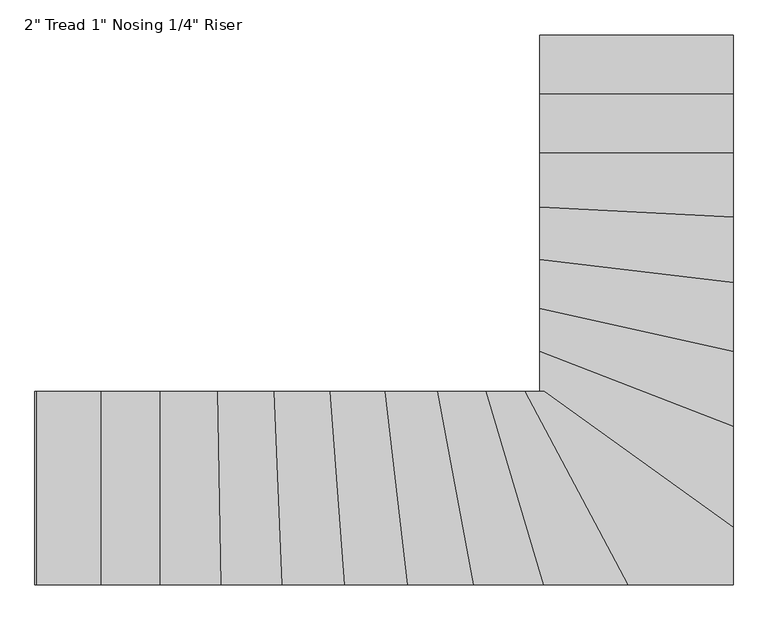
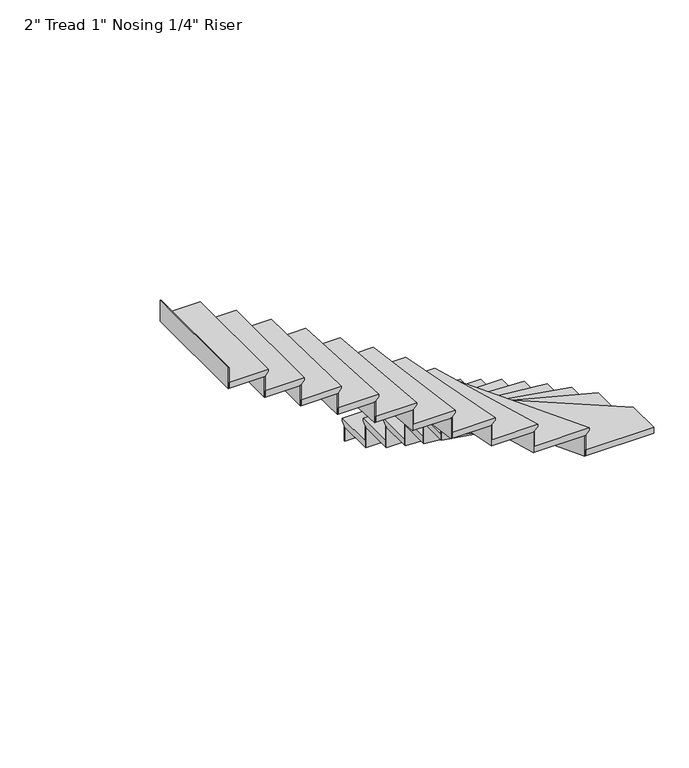
"""IFC4 building model written with IfcOpenShell, lengths in millimetres: stair flight geometry."""

from ifc_helpers import new_model, si_unit, origin, place, context, project, spatial, faceted_brep, source, transform, mapped, element, save


def stair_flight_9178a8c5(model_context):
    return source(origin(), model_context, "Body", "Brep", [
        faceted_brep([(541.8084916, 3870.4222402, 6551.0833333), (541.8084916, 3870.4222402, 6570.1333333), (1456.2084916, 3870.4222402, 6570.1333333), (1456.2084916, 3870.4222402, 6551.0833333), (541.8084916, 3845.0222402, 6525.6833333), (1456.2084916, 3845.0222402, 6525.6833333), (541.8084916, 3565.6222402, 6570.1333333), (1456.2084916, 3565.6222402, 6570.1333333), (1456.2084916, 3845.0222402, 6519.3333333), (1456.2084916, 3565.6222402, 6519.3333333), (541.8084916, 3565.6222402, 6519.3333333), (541.8084916, 3845.0222402, 6519.3333333)], [[[0, 1, 2, 3]], [[4, 0, 3, 5]], [[2, 1, 6, 7]], [[8, 9, 10, 11]], [[2, 7, 9, 8, 5, 3]], [[8, 11, 4, 5]], [[6, 1, 0, 4, 11, 10]], [[7, 6, 10, 9]]]),
        faceted_brep([(541.8084916, 3845.0222402, 6519.3333333), (541.8084916, 3845.0222402, 6400.8), (541.8084916, 3838.6722402, 6400.8), (541.8084916, 3838.6722402, 6519.3333333), (1456.2084916, 3845.0222402, 6519.3333333), (1456.2084916, 3838.6722402, 6519.3333333), (1456.2084916, 3838.6722402, 6400.8), (1456.2084916, 3845.0222402, 6400.8)], [[[0, 1, 2, 3]], [[4, 5, 6, 7]], [[1, 0, 4, 7]], [[2, 1, 7, 6]], [[3, 2, 6, 5]], [[0, 3, 5, 4]]]),
        faceted_brep([(541.8084916, 3565.6222402, 6688.6666667), (541.8084916, 3565.6222402, 6519.3333333), (541.8084916, 3559.2722402, 6519.3333333), (541.8084916, 3559.2722402, 6688.6666667), (1456.2084916, 3565.6222402, 6688.6666667), (1456.2084916, 3559.2722402, 6688.6666667), (1456.2084916, 3559.2722402, 6519.3333333), (1456.2084916, 3565.6222402, 6519.3333333)], [[[0, 1, 2, 3]], [[4, 5, 6, 7]], [[1, 0, 4, 7]], [[2, 1, 7, 6]], [[3, 2, 6, 5]], [[0, 3, 5, 4]]]),
        faceted_brep([(1456.2084916, 3591.0222402, 6739.4666667), (541.8084916, 3591.0222402, 6739.4666667), (541.8084916, 3286.2222402, 6739.4666667), (1456.2084916, 3286.2222402, 6739.4666667), (1456.2084916, 3565.6222402, 6688.6666667), (1456.2084916, 3286.2222402, 6688.6666667), (541.8084916, 3286.2222402, 6688.6666667), (541.8084916, 3565.6222402, 6688.6666667), (1456.2084916, 3565.6222402, 6695.0166667), (1456.2084916, 3591.0222402, 6720.4166667), (541.8084916, 3565.6222402, 6695.0166667), (541.8084916, 3591.0222402, 6720.4166667)], [[[0, 1, 2, 3]], [[4, 5, 6, 7]], [[0, 3, 5, 4, 8, 9]], [[4, 7, 10, 8]], [[2, 1, 11, 10, 7, 6]], [[3, 2, 6, 5]], [[11, 1, 0, 9]], [[10, 11, 9, 8]]]),
        faceted_brep([(541.8084916, 3286.2222402, 6858.0), (541.8084916, 3286.2222402, 6688.6666667), (541.8084916, 3279.8722402, 6688.6666667), (541.8084916, 3279.8722402, 6858.0), (1456.2084916, 3286.2222402, 6858.0), (1456.2084916, 3279.8722402, 6858.0), (1456.2084916, 3279.8722402, 6688.6666667), (1456.2084916, 3286.2222402, 6688.6666667)], [[[0, 1, 2, 3]], [[4, 5, 6, 7]], [[1, 0, 4, 7]], [[2, 1, 7, 6]], [[3, 2, 6, 5]], [[0, 3, 5, 4]]]),
        faceted_brep([(1456.2084916, 3311.6222402, 6908.8), (541.8084916, 3311.6222402, 6908.8), (541.8084916, 3029.9557204, 6908.8), (1456.2084916, 2983.6235901, 6908.8), (1456.2084916, 3286.2222402, 6858.0), (1456.2084916, 2983.6235901, 6858.0), (541.8084916, 3029.9557204, 6858.0), (541.8084916, 3286.2222402, 6858.0), (1456.2084916, 3286.2222402, 6864.35), (1456.2084916, 3311.6222402, 6889.75), (541.8084916, 3286.2222402, 6864.35), (541.8084916, 3311.6222402, 6889.75)], [[[0, 1, 2, 3]], [[4, 5, 6, 7]], [[0, 3, 5, 4, 8, 9]], [[4, 7, 10, 8]], [[2, 1, 11, 10, 7, 6]], [[3, 2, 6, 5]], [[11, 1, 0, 9]], [[10, 11, 9, 8]]]),
        faceted_brep([(541.8084916, 3029.9557204, 7027.3333333), (541.8084916, 3029.9557204, 6858.0), (541.8084916, 3023.5975741, 6858.0), (541.8084916, 3023.5975741, 7027.3333333), (1456.2084916, 2983.6235901, 7027.3333333), (1456.2084916, 2977.2654439, 7027.3333333), (1456.2084916, 2977.2654439, 6858.0), (1456.2084916, 2983.6235901, 6858.0)], [[[0, 1, 2, 3]], [[4, 5, 6, 7]], [[1, 0, 4, 7]], [[2, 1, 7, 6]], [[3, 2, 6, 5]], [[0, 3, 5, 4]]]),
        faceted_brep([(1456.2084916, 3009.0561751, 7078.1333333), (541.8084916, 3055.3883053, 7078.1333333), (541.8084916, 2782.3369776, 7078.1333333), (1456.2084916, 2672.1399389, 7078.1333333), (1456.2084916, 2983.6235901, 7027.3333333), (1456.2084916, 2672.1399389, 7027.3333333), (541.8084916, 2782.3369776, 7027.3333333), (541.8084916, 3029.9557204, 7027.3333333), (1456.2084916, 2983.6235901, 7033.6833333), (1456.2084916, 3009.0561751, 7059.0833333), (541.8084916, 3029.9557204, 7033.6833333), (541.8084916, 3055.3883053, 7059.0833333)], [[[0, 1, 2, 3]], [[4, 5, 6, 7]], [[0, 3, 5, 4, 8, 9]], [[4, 7, 10, 8]], [[2, 1, 11, 10, 7, 6]], [[3, 2, 6, 5]], [[11, 1, 0, 9]], [[10, 11, 9, 8]]]),
        faceted_brep([(541.8084916, 2782.3369776, 7196.6666667), (541.8084916, 2782.3369776, 7027.3333333), (541.8084916, 2775.9410322, 7027.3333333), (541.8084916, 2775.9410322, 7196.6666667), (1456.2084916, 2672.1399389, 7196.6666667), (1456.2084916, 2665.7439934, 7196.6666667), (1456.2084916, 2665.7439934, 7027.3333333), (1456.2084916, 2672.1399389, 7027.3333333)], [[[0, 1, 2, 3]], [[4, 5, 6, 7]], [[1, 0, 4, 7]], [[2, 1, 7, 6]], [[3, 2, 6, 5]], [[0, 3, 5, 4]]]),
        faceted_brep([(1456.2084916, 2697.7237208, 7247.4666667), (541.8084916, 2807.9207596, 7247.4666667), (541.8084916, 2549.3331683, 7247.4666667), (1456.2084916, 2345.4640286, 7247.4666667), (1456.2084916, 2672.1399389, 7196.6666667), (1456.2084916, 2345.4640286, 7196.6666667), (541.8084916, 2549.3331683, 7196.6666667), (541.8084916, 2782.3369776, 7196.6666667), (1456.2084916, 2672.1399389, 7203.0166667), (1456.2084916, 2697.7237208, 7228.4166667), (541.8084916, 2782.3369776, 7203.0166667), (541.8084916, 2807.9207596, 7228.4166667)], [[[0, 1, 2, 3]], [[4, 5, 6, 7]], [[0, 3, 5, 4, 8, 9]], [[4, 7, 10, 8]], [[2, 1, 11, 10, 7, 6]], [[3, 2, 6, 5]], [[11, 1, 0, 9]], [[10, 11, 9, 8]]]),
        faceted_brep([(541.8084916, 2549.3331683, 7366.0), (541.8084916, 2549.3331683, 7196.6666667), (541.8084916, 2542.8272579, 7196.6666667), (541.8084916, 2542.8272579, 7366.0), (1456.2084916, 2345.4640286, 7366.0), (1456.2084916, 2338.9581182, 7366.0), (1456.2084916, 2338.9581182, 7196.6666667), (1456.2084916, 2345.4640286, 7196.6666667)], [[[0, 1, 2, 3]], [[4, 5, 6, 7]], [[1, 0, 4, 7]], [[2, 1, 7, 6]], [[3, 2, 6, 5]], [[0, 3, 5, 4]]]),
        faceted_brep([(1456.2084916, 2371.4876703, 7416.8), (541.8084916, 2575.3568101, 7416.8), (541.8084916, 2344.0635087, 7416.8), (1456.2084916, 1989.4955623, 7416.8), (1456.2084916, 2345.4640286, 7366.0), (1456.2084916, 1989.4955623, 7366.0), (541.8084916, 2344.0635087, 7366.0), (541.8084916, 2549.3331683, 7366.0), (1456.2084916, 2345.4640286, 7372.35), (1456.2084916, 2371.4876703, 7397.75), (541.8084916, 2549.3331683, 7372.35), (541.8084916, 2575.3568101, 7397.75)], [[[0, 1, 2, 3]], [[4, 5, 6, 7]], [[0, 3, 5, 4, 8, 9]], [[4, 7, 10, 8]], [[2, 1, 11, 10, 7, 6]], [[3, 2, 6, 5]], [[11, 1, 0, 9]], [[10, 11, 9, 8]]]),
        faceted_brep([(541.8084916, 2344.0635087, 7535.3333333), (541.8084916, 2344.0635087, 7366.0), (541.8084916, 2337.2528325, 7366.0), (541.8084916, 2337.2528325, 7535.3333333), (1456.2084916, 1989.4955623, 7535.3333333), (1456.2084916, 1982.6848861, 7535.3333333), (1456.2084916, 1982.6848861, 7366.0), (1456.2084916, 1989.4955623, 7366.0)], [[[0, 1, 2, 3]], [[4, 5, 6, 7]], [[1, 0, 4, 7]], [[2, 1, 7, 6]], [[3, 2, 6, 5]], [[0, 3, 5, 4]]]),
        faceted_brep([(1456.2084916, 2016.738267, 7586.1333333), (541.8084916, 2371.3062134, 7586.1333333), (541.8084916, 2183.3652728, 7586.1333333), (518.7146085, 2183.3652728, 7586.1333333), (1456.2084916, 1508.8170155, 7586.1333333), (1456.2084916, 1989.4955623, 7535.3333333), (1456.2084916, 1508.8170155, 7535.3333333), (518.7146085, 2183.3652728, 7535.3333333), (541.8084916, 2183.3652728, 7535.3333333), (541.8084916, 2344.0635087, 7535.3333333), (1456.2084916, 1989.4955623, 7541.6833333), (1456.2084916, 2016.738267, 7567.0833333), (541.8084916, 2344.0635087, 7541.6833333), (541.8084916, 2371.3062134, 7567.0833333)], [[[0, 1, 2, 3, 4]], [[5, 6, 7, 8, 9]], [[0, 4, 6, 5, 10, 11]], [[5, 9, 12, 10]], [[2, 1, 13, 12, 9, 8]], [[4, 3, 7, 6]], [[13, 1, 0, 11]], [[12, 13, 11, 10]], [[3, 2, 8, 7]]]),
        faceted_brep([(518.7146085, 2183.3652728, 7704.6666667), (518.7146085, 2183.3652728, 7535.3333333), (507.8422444, 2183.3652728, 7535.3333333), (507.8422444, 2183.3652728, 7704.6666667), (1456.2084916, 1508.8170155, 7704.6666667), (1456.2084916, 1500.9941013, 7704.6666667), (1456.2084916, 1500.9941013, 7535.3333333), (1456.2084916, 1508.8170155, 7535.3333333)], [[[0, 1, 2, 3]], [[4, 5, 6, 7]], [[1, 0, 4, 7]], [[2, 1, 7, 6]], [[3, 2, 6, 5]], [[0, 3, 5, 4]]]),
        faceted_brep([(928.7056408, 1268.9652728, 7755.4666667), (1456.2084916, 1268.9652728, 7755.4666667), (1456.2084916, 1540.1086724, 7755.4666667), (562.2040648, 2183.3652728, 7755.4666667), (442.5531734, 2183.3652728, 7755.4666667), (1456.2084916, 1268.9652728, 7704.6666667), (928.7056408, 1268.9652728, 7704.6666667), (442.5531734, 2183.3652728, 7704.6666667), (518.7146085, 2183.3652728, 7704.6666667), (1456.2084916, 1508.8170155, 7704.6666667), (518.7146085, 2183.3652728, 7711.0166667), (1456.2084916, 1508.8170155, 7711.0166667), (562.2040648, 2183.3652728, 7736.4166667), (1456.2084916, 1540.1086724, 7736.4166667)], [[[0, 1, 2, 3, 4]], [[5, 6, 7, 8, 9]], [[1, 0, 6, 5]], [[9, 8, 10, 11]], [[0, 4, 7, 6]], [[12, 3, 2, 13]], [[10, 12, 13, 11]], [[2, 1, 5, 9, 11, 13]], [[4, 3, 12, 10, 8, 7]]]),
        faceted_brep([(442.5531734, 2183.3652728, 7874.0), (442.5531734, 2183.3652728, 7704.6666667), (435.3614926, 2183.3652728, 7704.6666667), (435.3614926, 2183.3652728, 7874.0), (928.7056408, 1268.9652728, 7874.0), (921.51396, 1268.9652728, 7874.0), (921.51396, 1268.9652728, 7704.6666667), (928.7056408, 1268.9652728, 7704.6666667)], [[[0, 1, 2, 3]], [[4, 5, 6, 7]], [[1, 0, 4, 7]], [[2, 1, 7, 6]], [[3, 2, 6, 5]], [[0, 3, 5, 4]]]),
        faceted_brep([(957.4723641, 1268.9652728, 7924.8), (471.3198967, 2183.3652728, 7924.8), (259.1852093, 2183.3652728, 7924.8), (530.810737, 1268.9652728, 7924.8), (928.7056408, 1268.9652728, 7874.0), (530.810737, 1268.9652728, 7874.0), (259.1852093, 2183.3652728, 7874.0), (442.5531734, 2183.3652728, 7874.0), (928.7056408, 1268.9652728, 7880.35), (957.4723641, 1268.9652728, 7905.75), (442.5531734, 2183.3652728, 7880.35), (471.3198967, 2183.3652728, 7905.75)], [[[0, 1, 2, 3]], [[4, 5, 6, 7]], [[0, 3, 5, 4, 8, 9]], [[4, 7, 10, 8]], [[2, 1, 11, 10, 7, 6]], [[3, 2, 6, 5]], [[11, 1, 0, 9]], [[10, 11, 9, 8]]]),
        faceted_brep([(259.1852093, 2183.3652728, 8043.3333333), (259.1852093, 2183.3652728, 7874.0), (252.5609672, 2183.3652728, 7874.0), (252.5609672, 2183.3652728, 8043.3333333), (530.810737, 1268.9652728, 8043.3333333), (524.1864949, 1268.9652728, 8043.3333333), (524.1864949, 1268.9652728, 7874.0), (530.810737, 1268.9652728, 7874.0)], [[[0, 1, 2, 3]], [[4, 5, 6, 7]], [[1, 0, 4, 7]], [[2, 1, 7, 6]], [[3, 2, 6, 5]], [[0, 3, 5, 4]]]),
        faceted_brep([(557.3077055, 1268.9652728, 8094.1333333), (285.6821779, 2183.3652728, 8094.1333333), (32.036519, 2183.3652728, 8094.1333333), (200.498444, 1268.9652728, 8094.1333333), (530.810737, 1268.9652728, 8043.3333333), (200.498444, 1268.9652728, 8043.3333333), (32.036519, 2183.3652728, 8043.3333333), (259.1852093, 2183.3652728, 8043.3333333), (530.810737, 1268.9652728, 8049.6833333), (557.3077055, 1268.9652728, 8075.0833333), (259.1852093, 2183.3652728, 8049.6833333), (285.6821779, 2183.3652728, 8075.0833333)], [[[0, 1, 2, 3]], [[4, 5, 6, 7]], [[0, 3, 5, 4, 8, 9]], [[4, 7, 10, 8]], [[2, 1, 11, 10, 7, 6]], [[3, 2, 6, 5]], [[11, 1, 0, 9]], [[10, 11, 9, 8]]]),
        faceted_brep([(32.036519, 2183.3652728, 8212.6666667), (32.036519, 2183.3652728, 8043.3333333), (25.579654, 2183.3652728, 8043.3333333), (25.579654, 2183.3652728, 8212.6666667), (200.498444, 1268.9652728, 8212.6666667), (194.0415789, 1268.9652728, 8212.6666667), (194.0415789, 1268.9652728, 8043.3333333), (200.498444, 1268.9652728, 8043.3333333)], [[[0, 1, 2, 3]], [[4, 5, 6, 7]], [[1, 0, 4, 7]], [[2, 1, 7, 6]], [[3, 2, 6, 5]], [[0, 3, 5, 4]]]),
        faceted_brep([(226.3259042, 1268.9652728, 8263.4666667), (57.8639792, 2183.3652728, 8263.4666667), (-216.5399099, 2183.3652728, 8263.4666667), (-109.2188993, 1268.9652728, 8263.4666667), (200.498444, 1268.9652728, 8212.6666667), (-109.2188993, 1268.9652728, 8212.6666667), (-216.5399099, 2183.3652728, 8212.6666667), (32.036519, 2183.3652728, 8212.6666667), (200.498444, 1268.9652728, 8219.0166667), (226.3259042, 1268.9652728, 8244.4166667), (32.036519, 2183.3652728, 8219.0166667), (57.8639792, 2183.3652728, 8244.4166667)], [[[0, 1, 2, 3]], [[4, 5, 6, 7]], [[0, 3, 5, 4, 8, 9]], [[4, 7, 10, 8]], [[2, 1, 11, 10, 7, 6]], [[3, 2, 6, 5]], [[11, 1, 0, 9]], [[10, 11, 9, 8]]]),
        faceted_brep([(-216.5399099, 2183.3652728, 8382.0), (-216.5399099, 2183.3652728, 8212.6666667), (-222.9334965, 2183.3652728, 8212.6666667), (-222.9334965, 2183.3652728, 8382.0), (-109.2188993, 1268.9652728, 8382.0), (-115.6124859, 1268.9652728, 8382.0), (-115.6124859, 1268.9652728, 8212.6666667), (-109.2188993, 1268.9652728, 8212.6666667)], [[[0, 1, 2, 3]], [[4, 5, 6, 7]], [[1, 0, 4, 7]], [[2, 1, 7, 6]], [[3, 2, 6, 5]], [[0, 3, 5, 4]]]),
        faceted_brep([(-83.644553, 1268.9652728, 8432.8), (-190.9655636, 2183.3652728, 8432.8), (-475.6084446, 2183.3652728, 8432.8), (-408.7373342, 1268.9652728, 8432.8), (-109.2188993, 1268.9652728, 8382.0), (-408.7373342, 1268.9652728, 8382.0), (-475.6084446, 2183.3652728, 8382.0), (-216.5399099, 2183.3652728, 8382.0), (-109.2188993, 1268.9652728, 8388.35), (-83.644553, 1268.9652728, 8413.75), (-216.5399099, 2183.3652728, 8388.35), (-190.9655636, 2183.3652728, 8413.75)], [[[0, 1, 2, 3]], [[4, 5, 6, 7]], [[0, 3, 5, 4, 8, 9]], [[4, 7, 10, 8]], [[2, 1, 11, 10, 7, 6]], [[3, 2, 6, 5]], [[11, 1, 0, 9]], [[10, 11, 9, 8]]]),
        faceted_brep([(-475.6084446, 2183.3652728, 8551.3333333), (-475.6084446, 2183.3652728, 8382.0), (-481.9754023, 2183.3652728, 8382.0), (-481.9754023, 2183.3652728, 8551.3333333), (-408.7373342, 1268.9652728, 8551.3333333), (-415.104292, 1268.9652728, 8551.3333333), (-415.104292, 1268.9652728, 8382.0), (-408.7373342, 1268.9652728, 8382.0)], [[[0, 1, 2, 3]], [[4, 5, 6, 7]], [[1, 0, 4, 7]], [[2, 1, 7, 6]], [[3, 2, 6, 5]], [[0, 3, 5, 4]]]),
        faceted_brep([(-383.2695031, 1268.9652728, 8602.1333333), (-450.1406135, 2183.3652728, 8602.1333333), (-740.5916411, 2183.3652728, 8602.1333333), (-702.4626207, 1268.9652728, 8602.1333333), (-408.7373342, 1268.9652728, 8551.3333333), (-702.4626207, 1268.9652728, 8551.3333333), (-740.5916411, 2183.3652728, 8551.3333333), (-475.6084446, 2183.3652728, 8551.3333333), (-408.7373342, 1268.9652728, 8557.6833333), (-383.2695031, 1268.9652728, 8583.0833333), (-475.6084446, 2183.3652728, 8557.6833333), (-450.1406135, 2183.3652728, 8583.0833333)], [[[0, 1, 2, 3]], [[4, 5, 6, 7]], [[0, 3, 5, 4, 8, 9]], [[4, 7, 10, 8]], [[2, 1, 11, 10, 7, 6]], [[3, 2, 6, 5]], [[11, 1, 0, 9]], [[10, 11, 9, 8]]]),
        faceted_brep([(-740.5916411, 2183.3652728, 8720.6666667), (-740.5916411, 2183.3652728, 8551.3333333), (-746.9471593, 2183.3652728, 8551.3333333), (-746.9471593, 2183.3652728, 8720.6666667), (-702.4626207, 1268.9652728, 8720.6666667), (-708.8181389, 1268.9652728, 8720.6666667), (-708.8181389, 1268.9652728, 8551.3333333), (-702.4626207, 1268.9652728, 8551.3333333)], [[[0, 1, 2, 3]], [[4, 5, 6, 7]], [[1, 0, 4, 7]], [[2, 1, 7, 6]], [[3, 2, 6, 5]], [[0, 3, 5, 4]]]),
        faceted_brep([(-677.0405481, 1268.9652728, 8771.4666667), (-715.1695685, 2183.3652728, 8771.4666667), (-1009.2364216, 2183.3652728, 8771.4666667), (-992.5821201, 1268.9652728, 8771.4666667), (-702.4626207, 1268.9652728, 8720.6666667), (-992.5821201, 1268.9652728, 8720.6666667), (-1009.2364216, 2183.3652728, 8720.6666667), (-740.5916411, 2183.3652728, 8720.6666667), (-702.4626207, 1268.9652728, 8727.0166667), (-677.0405481, 1268.9652728, 8752.4166667), (-740.5916411, 2183.3652728, 8727.0166667), (-715.1695685, 2183.3652728, 8752.4166667)], [[[0, 1, 2, 3]], [[4, 5, 6, 7]], [[0, 3, 5, 4, 8, 9]], [[4, 7, 10, 8]], [[2, 1, 11, 10, 7, 6]], [[3, 2, 6, 5]], [[11, 1, 0, 9]], [[10, 11, 9, 8]]]),
        faceted_brep([(-1009.2364216, 2183.3652728, 8890.0), (-1009.2364216, 2183.3652728, 8720.6666667), (-1015.5874748, 2183.3652728, 8720.6666667), (-1015.5874748, 2183.3652728, 8890.0), (-992.5821201, 1268.9652728, 8890.0), (-998.9331733, 1268.9652728, 8890.0), (-998.9331733, 1268.9652728, 8720.6666667), (-992.5821201, 1268.9652728, 8720.6666667)], [[[0, 1, 2, 3]], [[4, 5, 6, 7]], [[1, 0, 4, 7]], [[2, 1, 7, 6]], [[3, 2, 6, 5]], [[0, 3, 5, 4]]]),
        faceted_brep([(-967.1779075, 1268.9652728, 8940.8), (-983.832209, 2183.3652728, 8940.8), (-1280.3050583, 2183.3652728, 8940.8), (-1280.3050583, 1268.9652728, 8940.8), (-992.5821201, 1268.9652728, 8890.0), (-1280.3050583, 1268.9652728, 8890.0), (-1280.3050583, 2183.3652728, 8890.0), (-1009.2364216, 2183.3652728, 8890.0), (-992.5821201, 1268.9652728, 8896.35), (-967.1779075, 1268.9652728, 8921.75), (-1009.2364216, 2183.3652728, 8896.35), (-983.832209, 2183.3652728, 8921.75)], [[[0, 1, 2, 3]], [[4, 5, 6, 7]], [[0, 3, 5, 4, 8, 9]], [[4, 7, 10, 8]], [[2, 1, 11, 10, 7, 6]], [[3, 2, 6, 5]], [[11, 1, 0, 9]], [[10, 11, 9, 8]]]),
        faceted_brep([(-1280.3050583, 2183.3652728, 9059.3333333), (-1280.3050583, 2183.3652728, 8890.0), (-1286.6550583, 2183.3652728, 8890.0), (-1286.6550583, 2183.3652728, 9059.3333333), (-1280.3050583, 1268.9652728, 9059.3333333), (-1286.6550583, 1268.9652728, 9059.3333333), (-1286.6550583, 1268.9652728, 8890.0), (-1280.3050583, 1268.9652728, 8890.0)], [[[0, 1, 2, 3]], [[4, 5, 6, 7]], [[1, 0, 4, 7]], [[2, 1, 7, 6]], [[3, 2, 6, 5]], [[0, 3, 5, 4]]]),
        faceted_brep([(-1254.9050583, 1268.9652728, 9110.1333333), (-1254.9050583, 2183.3652728, 9110.1333333), (-1559.7050583, 2183.3652728, 9110.1333333), (-1559.7050583, 1268.9652728, 9110.1333333), (-1280.3050583, 1268.9652728, 9059.3333333), (-1559.7050583, 1268.9652728, 9059.3333333), (-1559.7050583, 2183.3652728, 9059.3333333), (-1280.3050583, 2183.3652728, 9059.3333333), (-1280.3050583, 1268.9652728, 9065.6833333), (-1254.9050583, 1268.9652728, 9091.0833333), (-1280.3050583, 2183.3652728, 9065.6833333), (-1254.9050583, 2183.3652728, 9091.0833333)], [[[0, 1, 2, 3]], [[4, 5, 6, 7]], [[0, 3, 5, 4, 8, 9]], [[4, 7, 10, 8]], [[2, 1, 11, 10, 7, 6]], [[3, 2, 6, 5]], [[11, 1, 0, 9]], [[10, 11, 9, 8]]]),
        faceted_brep([(-1559.7050583, 2183.3652728, 9228.6666667), (-1559.7050583, 2183.3652728, 9059.3333333), (-1566.0550583, 2183.3652728, 9059.3333333), (-1566.0550583, 2183.3652728, 9228.6666667), (-1559.7050583, 1268.9652728, 9228.6666667), (-1566.0550583, 1268.9652728, 9228.6666667), (-1566.0550583, 1268.9652728, 9059.3333333), (-1559.7050583, 1268.9652728, 9059.3333333)], [[[0, 1, 2, 3]], [[4, 5, 6, 7]], [[1, 0, 4, 7]], [[2, 1, 7, 6]], [[3, 2, 6, 5]], [[0, 3, 5, 4]]]),
        faceted_brep([(-1839.1050583, 2183.3652728, 9398.0), (-1839.1050583, 2183.3652728, 9228.6666667), (-1845.4550583, 2183.3652728, 9228.6666667), (-1845.4550583, 2183.3652728, 9398.0), (-1839.1050583, 1268.9652728, 9398.0), (-1845.4550583, 1268.9652728, 9398.0), (-1845.4550583, 1268.9652728, 9228.6666667), (-1839.1050583, 1268.9652728, 9228.6666667)], [[[0, 1, 2, 3]], [[4, 5, 6, 7]], [[1, 0, 4, 7]], [[2, 1, 7, 6]], [[3, 2, 6, 5]], [[0, 3, 5, 4]]]),
        faceted_brep([(-1534.3050583, 1268.9652728, 9279.4666667), (-1534.3050583, 2183.3652728, 9279.4666667), (-1839.1050583, 2183.3652728, 9279.4666667), (-1839.1050583, 1268.9652728, 9279.4666667), (-1559.7050583, 1268.9652728, 9228.6666667), (-1839.1050583, 1268.9652728, 9228.6666667), (-1839.1050583, 2183.3652728, 9228.6666667), (-1559.7050583, 2183.3652728, 9228.6666667), (-1559.7050583, 1268.9652728, 9235.0166667), (-1534.3050583, 1268.9652728, 9260.4166667), (-1559.7050583, 2183.3652728, 9235.0166667), (-1534.3050583, 2183.3652728, 9260.4166667)], [[[0, 1, 2, 3]], [[4, 5, 6, 7]], [[0, 3, 5, 4, 8, 9]], [[4, 7, 10, 8]], [[2, 1, 11, 10, 7, 6]], [[3, 2, 6, 5]], [[11, 1, 0, 9]], [[10, 11, 9, 8]]]),
    ])


if __name__ == "__main__":
    model = new_model("IFC4")
    model_context = context("Model", 3, world=origin())
    ifc_project = project(units=[si_unit("LENGTHUNIT", "METRE", prefix="MILLI")], contexts=[model_context])
    site = spatial("IfcSite", under=ifc_project)
    building = spatial("IfcBuilding", under=site)
    placement = place(None, origin())
    stair_flight_shape = stair_flight_9178a8c5(model_context)
    element("IfcStairFlight", 1, ObjectType="2\" Tread 1\" Nosing 1/4\" Riser", at=placement, inside=building, context=model_context, shape_type="MappedRepresentation", body=[
        mapped(stair_flight_shape, transform((0.0, 0.0, 0.0), x_axis=(1.0, 0.0, 0.0), y_axis=(0.0, 1.0, 0.0), z_axis=(0.0, 0.0, 1.0))),
    ])
    save(model, "model.ifc")
